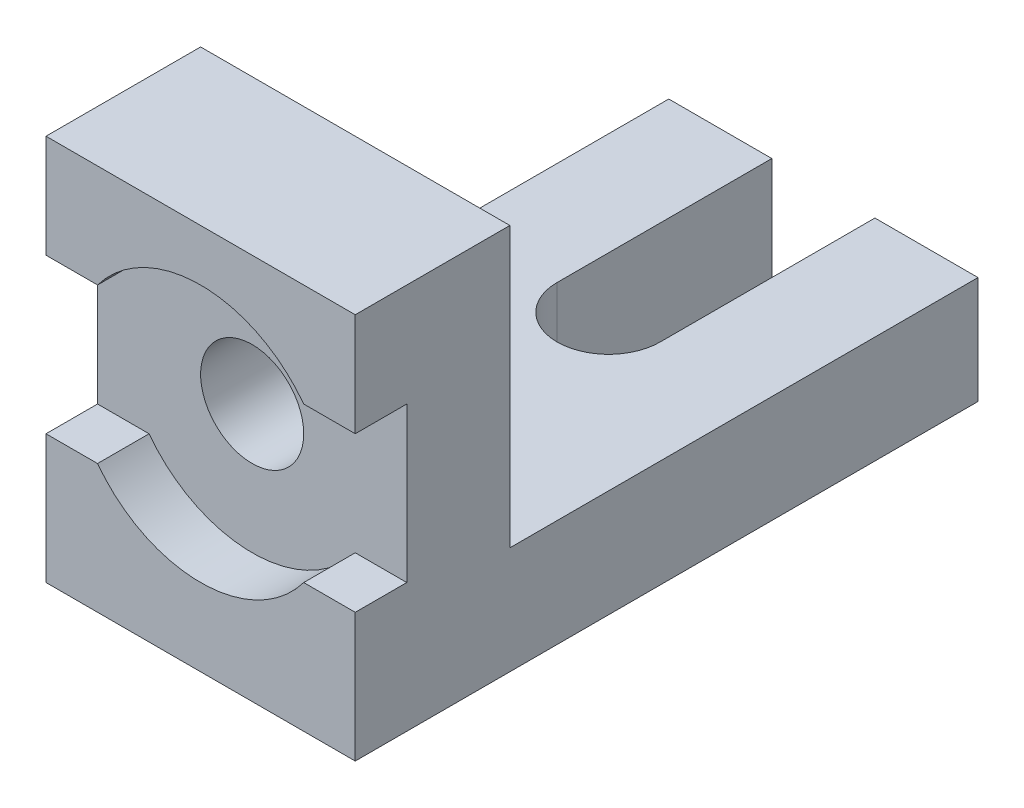
ISO-10303-21;
HEADER;
FILE_DESCRIPTION(('STEP AP214'),'2;1');
FILE_NAME('part.step','',(''),(''),'','','');
FILE_SCHEMA(('AUTOMOTIVE_DESIGN { 1 0 10303 214 1 1 1 1 }'));
ENDSEC;
DATA;
#1=APPLICATION_CONTEXT('core data for automotive mechanical design processes');
#2=APPLICATION_PROTOCOL_DEFINITION('international standard','automotive_design',2000,#1);
#3=PRODUCT_CONTEXT('',#1,'mechanical');
#4=PRODUCT('Part','Part','',(#3));
#5=PRODUCT_RELATED_PRODUCT_CATEGORY('part','',(#4));
#6=PRODUCT_DEFINITION_FORMATION('','',#4);
#7=PRODUCT_DEFINITION_CONTEXT('part definition',#1,'design');
#8=PRODUCT_DEFINITION('design','',#6,#7);
#9=PRODUCT_DEFINITION_SHAPE('','',#8);
#10=(LENGTH_UNIT() NAMED_UNIT(*) SI_UNIT(.MILLI.,.METRE.));
#11=(NAMED_UNIT(*) PLANE_ANGLE_UNIT() SI_UNIT($,.RADIAN.));
#12=(NAMED_UNIT(*) SI_UNIT($,.STERADIAN.) SOLID_ANGLE_UNIT());
#13=UNCERTAINTY_MEASURE_WITH_UNIT(LENGTH_MEASURE(1.E-05),#10,'distance_accuracy_value','');
#14=(GEOMETRIC_REPRESENTATION_CONTEXT(3) GLOBAL_UNCERTAINTY_ASSIGNED_CONTEXT((#13)) GLOBAL_UNIT_ASSIGNED_CONTEXT((#10,
#11,#12)) REPRESENTATION_CONTEXT('',''));
#15=CARTESIAN_POINT('',(0.,0.,0.));
#16=DIRECTION('',(0.,0.,1.));
#17=DIRECTION('',(1.,0.,0.));
#18=AXIS2_PLACEMENT_3D('',#15,#16,#17);
#19=CARTESIAN_POINT('',(-36.,25.,72.5));
#20=DIRECTION('',(0.,0.,-1.));
#21=DIRECTION('',(-1.,0.,0.));
#22=AXIS2_PLACEMENT_3D('',#19,#20,#21);
#23=PLANE('',#22);
#24=DIRECTION('',(0.,-1.,0.));
#25=VECTOR('',#24,1.);
#26=CARTESIAN_POINT('',(-36.,25.,72.5));
#27=LINE('',#26,#25);
#28=CARTESIAN_POINT('',(-36.,90.,72.5));
#29=VERTEX_POINT('',#28);
#30=CARTESIAN_POINT('',(-36.,66.,72.5));
#31=VERTEX_POINT('',#30);
#32=EDGE_CURVE('E288',#29,#31,#27,.T.);
#33=ORIENTED_EDGE('',*,*,#32,.T.);
#34=DIRECTION('',(-1.,0.,0.));
#35=VECTOR('',#34,1.);
#36=CARTESIAN_POINT('',(0.,66.,72.5));
#37=LINE('',#36,#35);
#38=CARTESIAN_POINT('',(-24.,66.,72.5));
#39=VERTEX_POINT('',#38);
#40=EDGE_CURVE('E183',#39,#31,#37,.T.);
#41=ORIENTED_EDGE('',*,*,#40,.F.);
#42=CARTESIAN_POINT('',(0.,48.,72.5));
#43=DIRECTION('',(0.,0.,1.));
#44=DIRECTION('',(1.,0.,0.));
#45=AXIS2_PLACEMENT_3D('',#42,#43,#44);
#46=CIRCLE('',#45,30.);
#47=CARTESIAN_POINT('',(24.,66.,72.5));
#48=VERTEX_POINT('',#47);
#49=EDGE_CURVE('E190',#48,#39,#46,.T.);
#50=ORIENTED_EDGE('',*,*,#49,.F.);
#51=DIRECTION('',(-1.,0.,0.));
#52=VECTOR('',#51,1.);
#53=CARTESIAN_POINT('',(0.,66.,72.5));
#54=LINE('',#53,#52);
#55=CARTESIAN_POINT('',(36.,66.,72.5));
#56=VERTEX_POINT('',#55);
#57=EDGE_CURVE('E211',#56,#48,#54,.T.);
#58=ORIENTED_EDGE('',*,*,#57,.F.);
#59=DIRECTION('',(0.,-1.,0.));
#60=VECTOR('',#59,1.);
#61=CARTESIAN_POINT('',(36.,25.,72.5));
#62=LINE('',#61,#60);
#63=CARTESIAN_POINT('',(36.,90.,72.5));
#64=VERTEX_POINT('',#63);
#65=EDGE_CURVE('E287',#64,#56,#62,.T.);
#66=ORIENTED_EDGE('',*,*,#65,.F.);
#67=DIRECTION('',(1.,0.,0.));
#68=VECTOR('',#67,1.);
#69=CARTESIAN_POINT('',(-36.,90.,72.5));
#70=LINE('',#69,#68);
#71=EDGE_CURVE('E232',#29,#64,#70,.T.);
#72=ORIENTED_EDGE('',*,*,#71,.F.);
#73=EDGE_LOOP('',(#33,#41,#50,#58,#66,#72));
#74=FACE_BOUND('',#73,.T.);
#75=ADVANCED_FACE('F39',(#74),#23,.F.);
#76=CARTESIAN_POINT('',(36.,25.,-72.5));
#77=DIRECTION('',(0.,0.,1.));
#78=DIRECTION('',(1.,0.,0.));
#79=AXIS2_PLACEMENT_3D('',#76,#77,#78);
#80=PLANE('',#79);
#81=DIRECTION('',(-1.,0.,0.));
#82=VECTOR('',#81,1.);
#83=CARTESIAN_POINT('',(36.,25.,-72.5));
#84=LINE('',#83,#82);
#85=CARTESIAN_POINT('',(-12.,25.,-72.5));
#86=VERTEX_POINT('',#85);
#87=CARTESIAN_POINT('',(-36.,25.,-72.5));
#88=VERTEX_POINT('',#87);
#89=EDGE_CURVE('E268',#86,#88,#84,.T.);
#90=ORIENTED_EDGE('',*,*,#89,.F.);
#91=DIRECTION('',(0.,1.,0.));
#92=VECTOR('',#91,1.);
#93=CARTESIAN_POINT('',(-12.,-25.,-72.5));
#94=LINE('',#93,#92);
#95=CARTESIAN_POINT('',(-12.,0.,-72.5));
#96=VERTEX_POINT('',#95);
#97=EDGE_CURVE('E257',#96,#86,#94,.T.);
#98=ORIENTED_EDGE('',*,*,#97,.F.);
#99=DIRECTION('',(-1.,0.,0.));
#100=VECTOR('',#99,1.);
#101=CARTESIAN_POINT('',(36.,0.,-72.5));
#102=LINE('',#101,#100);
#103=CARTESIAN_POINT('',(-36.,0.,-72.5));
#104=VERTEX_POINT('',#103);
#105=EDGE_CURVE('E280',#96,#104,#102,.T.);
#106=ORIENTED_EDGE('',*,*,#105,.T.);
#107=DIRECTION('',(0.,-1.,0.));
#108=VECTOR('',#107,1.);
#109=CARTESIAN_POINT('',(-36.,25.,-72.5));
#110=LINE('',#109,#108);
#111=EDGE_CURVE('E291',#88,#104,#110,.T.);
#112=ORIENTED_EDGE('',*,*,#111,.F.);
#113=EDGE_LOOP('',(#90,#98,#106,#112));
#114=FACE_BOUND('',#113,.T.);
#115=ADVANCED_FACE('F338',(#114),#80,.F.);
#116=CARTESIAN_POINT('',(36.,25.,0.));
#117=DIRECTION('',(-1.,0.,0.));
#118=DIRECTION('',(0.,0.,1.));
#119=AXIS2_PLACEMENT_3D('',#116,#117,#118);
#120=PLANE('',#119);
#121=ORIENTED_EDGE('',*,*,#65,.T.);
#122=DIRECTION('',(0.,0.,1.));
#123=VECTOR('',#122,1.);
#124=CARTESIAN_POINT('',(36.,66.,60.5));
#125=LINE('',#124,#123);
#126=CARTESIAN_POINT('',(36.,66.,60.5));
#127=VERTEX_POINT('',#126);
#128=EDGE_CURVE('E223',#127,#56,#125,.T.);
#129=ORIENTED_EDGE('',*,*,#128,.F.);
#130=DIRECTION('',(0.,1.,0.));
#131=VECTOR('',#130,1.);
#132=CARTESIAN_POINT('',(36.,0.,60.5));
#133=LINE('',#132,#131);
#134=CARTESIAN_POINT('',(36.,30.,60.5));
#135=VERTEX_POINT('',#134);
#136=EDGE_CURVE('E191',#135,#127,#133,.T.);
#137=ORIENTED_EDGE('',*,*,#136,.F.);
#138=DIRECTION('',(0.,0.,1.));
#139=VECTOR('',#138,1.);
#140=CARTESIAN_POINT('',(36.,30.,60.5));
#141=LINE('',#140,#139);
#142=CARTESIAN_POINT('',(36.,30.,72.5));
#143=VERTEX_POINT('',#142);
#144=EDGE_CURVE('E230',#135,#143,#141,.T.);
#145=ORIENTED_EDGE('',*,*,#144,.T.);
#146=CARTESIAN_POINT('',(36.,0.,72.5));
#147=VERTEX_POINT('',#146);
#148=EDGE_CURVE('E274',#143,#147,#62,.T.);
#149=ORIENTED_EDGE('',*,*,#148,.T.);
#150=DIRECTION('',(0.,0.,-1.));
#151=VECTOR('',#150,1.);
#152=CARTESIAN_POINT('',(36.,0.,0.));
#153=LINE('',#152,#151);
#154=CARTESIAN_POINT('',(36.,0.,-72.5));
#155=VERTEX_POINT('',#154);
#156=EDGE_CURVE('E259',#147,#155,#153,.T.);
#157=ORIENTED_EDGE('',*,*,#156,.T.);
#158=DIRECTION('',(0.,-1.,0.));
#159=VECTOR('',#158,1.);
#160=CARTESIAN_POINT('',(36.,25.,-72.5));
#161=LINE('',#160,#159);
#162=CARTESIAN_POINT('',(36.,25.,-72.5));
#163=VERTEX_POINT('',#162);
#164=EDGE_CURVE('E297',#163,#155,#161,.T.);
#165=ORIENTED_EDGE('',*,*,#164,.F.);
#166=DIRECTION('',(0.,0.,-1.));
#167=VECTOR('',#166,1.);
#168=CARTESIAN_POINT('',(36.,25.,72.5));
#169=LINE('',#168,#167);
#170=CARTESIAN_POINT('',(36.,25.,36.5));
#171=VERTEX_POINT('',#170);
#172=EDGE_CURVE('E266',#171,#163,#169,.T.);
#173=ORIENTED_EDGE('',*,*,#172,.F.);
#174=DIRECTION('',(0.,-1.,0.));
#175=VECTOR('',#174,1.);
#176=CARTESIAN_POINT('',(36.,90.,36.5));
#177=LINE('',#176,#175);
#178=CARTESIAN_POINT('',(36.,90.,36.5));
#179=VERTEX_POINT('',#178);
#180=EDGE_CURVE('E241',#179,#171,#177,.T.);
#181=ORIENTED_EDGE('',*,*,#180,.F.);
#182=DIRECTION('',(0.,0.,-1.));
#183=VECTOR('',#182,1.);
#184=CARTESIAN_POINT('',(36.,90.,72.5));
#185=LINE('',#184,#183);
#186=EDGE_CURVE('E231',#64,#179,#185,.T.);
#187=ORIENTED_EDGE('',*,*,#186,.F.);
#188=EDGE_LOOP('',(#121,#129,#137,#145,#149,#157,#165,#173,#181,#187));
#189=FACE_BOUND('',#188,.T.);
#190=ADVANCED_FACE('F41',(#189),#120,.F.);
#191=CARTESIAN_POINT('',(12.,0.,-72.5));
#192=VERTEX_POINT('',#191);
#193=EDGE_CURVE('E279',#155,#192,#102,.T.);
#194=ORIENTED_EDGE('',*,*,#193,.T.);
#195=DIRECTION('',(0.,1.,0.));
#196=VECTOR('',#195,1.);
#197=CARTESIAN_POINT('',(12.,-25.,-72.5));
#198=LINE('',#197,#196);
#199=CARTESIAN_POINT('',(12.,25.,-72.5));
#200=VERTEX_POINT('',#199);
#201=EDGE_CURVE('E265',#192,#200,#198,.T.);
#202=ORIENTED_EDGE('',*,*,#201,.T.);
#203=EDGE_CURVE('E269',#163,#200,#84,.T.);
#204=ORIENTED_EDGE('',*,*,#203,.F.);
#205=ORIENTED_EDGE('',*,*,#164,.T.);
#206=EDGE_LOOP('',(#194,#202,#204,#205));
#207=FACE_BOUND('',#206,.T.);
#208=ADVANCED_FACE('F325',(#207),#80,.F.);
#209=CARTESIAN_POINT('',(-36.,25.,-72.5));
#210=DIRECTION('',(1.,0.,0.));
#211=DIRECTION('',(0.,0.,-1.));
#212=AXIS2_PLACEMENT_3D('',#209,#210,#211);
#213=PLANE('',#212);
#214=CARTESIAN_POINT('',(-36.,30.,72.5));
#215=VERTEX_POINT('',#214);
#216=CARTESIAN_POINT('',(-36.,0.,72.5));
#217=VERTEX_POINT('',#216);
#218=EDGE_CURVE('E286',#215,#217,#27,.T.);
#219=ORIENTED_EDGE('',*,*,#218,.F.);
#220=DIRECTION('',(0.,0.,1.));
#221=VECTOR('',#220,1.);
#222=CARTESIAN_POINT('',(-36.,30.,60.5));
#223=LINE('',#222,#221);
#224=CARTESIAN_POINT('',(-36.,30.,60.5));
#225=VERTEX_POINT('',#224);
#226=EDGE_CURVE('E216',#225,#215,#223,.T.);
#227=ORIENTED_EDGE('',*,*,#226,.F.);
#228=DIRECTION('',(0.,-1.,0.));
#229=VECTOR('',#228,1.);
#230=CARTESIAN_POINT('',(-36.,0.,60.5));
#231=LINE('',#230,#229);
#232=CARTESIAN_POINT('',(-36.,66.,60.5));
#233=VERTEX_POINT('',#232);
#234=EDGE_CURVE('E172',#233,#225,#231,.T.);
#235=ORIENTED_EDGE('',*,*,#234,.F.);
#236=DIRECTION('',(0.,0.,1.));
#237=VECTOR('',#236,1.);
#238=CARTESIAN_POINT('',(-36.,66.,60.5));
#239=LINE('',#238,#237);
#240=EDGE_CURVE('E217',#233,#31,#239,.T.);
#241=ORIENTED_EDGE('',*,*,#240,.T.);
#242=ORIENTED_EDGE('',*,*,#32,.F.);
#243=DIRECTION('',(0.,0.,1.));
#244=VECTOR('',#243,1.);
#245=CARTESIAN_POINT('',(-36.,90.,36.5));
#246=LINE('',#245,#244);
#247=CARTESIAN_POINT('',(-36.,90.,36.5));
#248=VERTEX_POINT('',#247);
#249=EDGE_CURVE('E236',#248,#29,#246,.T.);
#250=ORIENTED_EDGE('',*,*,#249,.F.);
#251=DIRECTION('',(0.,-1.,0.));
#252=VECTOR('',#251,1.);
#253=CARTESIAN_POINT('',(-36.,90.,36.5));
#254=LINE('',#253,#252);
#255=CARTESIAN_POINT('',(-36.,25.,36.5));
#256=VERTEX_POINT('',#255);
#257=EDGE_CURVE('E242',#248,#256,#254,.T.);
#258=ORIENTED_EDGE('',*,*,#257,.T.);
#259=DIRECTION('',(0.,0.,1.));
#260=VECTOR('',#259,1.);
#261=CARTESIAN_POINT('',(-36.,25.,-72.5));
#262=LINE('',#261,#260);
#263=EDGE_CURVE('E272',#88,#256,#262,.T.);
#264=ORIENTED_EDGE('',*,*,#263,.F.);
#265=ORIENTED_EDGE('',*,*,#111,.T.);
#266=DIRECTION('',(0.,0.,1.));
#267=VECTOR('',#266,1.);
#268=CARTESIAN_POINT('',(-36.,0.,-72.5));
#269=LINE('',#268,#267);
#270=EDGE_CURVE('E282',#104,#217,#269,.T.);
#271=ORIENTED_EDGE('',*,*,#270,.T.);
#272=EDGE_LOOP('',(#219,#227,#235,#241,#242,#250,#258,#264,#265,#271));
#273=FACE_BOUND('',#272,.T.);
#274=ADVANCED_FACE('F331',(#273),#213,.F.);
#275=CARTESIAN_POINT('',(0.,48.,72.5));
#276=DIRECTION('',(0.,0.,1.));
#277=DIRECTION('',(1.,0.,0.));
#278=AXIS2_PLACEMENT_3D('',#275,#276,#277);
#279=CIRCLE('',#278,30.);
#280=CARTESIAN_POINT('',(-24.,30.,72.5));
#281=VERTEX_POINT('',#280);
#282=CARTESIAN_POINT('',(24.,30.,72.5));
#283=VERTEX_POINT('',#282);
#284=EDGE_CURVE('E210',#281,#283,#279,.T.);
#285=ORIENTED_EDGE('',*,*,#284,.F.);
#286=DIRECTION('',(1.,0.,0.));
#287=VECTOR('',#286,1.);
#288=CARTESIAN_POINT('',(0.,30.,72.5));
#289=LINE('',#288,#287);
#290=EDGE_CURVE('E53',#215,#281,#289,.T.);
#291=ORIENTED_EDGE('',*,*,#290,.F.);
#292=ORIENTED_EDGE('',*,*,#218,.T.);
#293=DIRECTION('',(1.,0.,0.));
#294=VECTOR('',#293,1.);
#295=CARTESIAN_POINT('',(-36.,0.,72.5));
#296=LINE('',#295,#294);
#297=EDGE_CURVE('E267',#217,#147,#296,.T.);
#298=ORIENTED_EDGE('',*,*,#297,.T.);
#299=ORIENTED_EDGE('',*,*,#148,.F.);
#300=DIRECTION('',(1.,0.,0.));
#301=VECTOR('',#300,1.);
#302=CARTESIAN_POINT('',(0.,30.,72.5));
#303=LINE('',#302,#301);
#304=EDGE_CURVE('E207',#283,#143,#303,.T.);
#305=ORIENTED_EDGE('',*,*,#304,.F.);
#306=EDGE_LOOP('',(#285,#291,#292,#298,#299,#305));
#307=FACE_BOUND('',#306,.T.);
#308=ADVANCED_FACE('F329',(#307),#23,.F.);
#309=CARTESIAN_POINT('',(0.,25.,0.));
#310=DIRECTION('',(0.,1.,0.));
#311=DIRECTION('',(0.,0.,1.));
#312=AXIS2_PLACEMENT_3D('',#309,#310,#311);
#313=PLANE('',#312);
#314=DIRECTION('',(-1.,0.,0.));
#315=VECTOR('',#314,1.);
#316=CARTESIAN_POINT('',(36.,25.,36.5));
#317=LINE('',#316,#315);
#318=EDGE_CURVE('E65',#171,#256,#317,.T.);
#319=ORIENTED_EDGE('',*,*,#318,.F.);
#320=ORIENTED_EDGE('',*,*,#172,.T.);
#321=ORIENTED_EDGE('',*,*,#203,.T.);
#322=DIRECTION('',(0.,0.,-1.));
#323=VECTOR('',#322,1.);
#324=CARTESIAN_POINT('',(12.,25.,-22.5));
#325=LINE('',#324,#323);
#326=CARTESIAN_POINT('',(12.,25.,-22.5));
#327=VERTEX_POINT('',#326);
#328=EDGE_CURVE('E253',#327,#200,#325,.T.);
#329=ORIENTED_EDGE('',*,*,#328,.F.);
#330=CARTESIAN_POINT('',(0.,25.,-22.5));
#331=DIRECTION('',(0.,1.,0.));
#332=DIRECTION('',(0.,0.,1.));
#333=AXIS2_PLACEMENT_3D('',#330,#331,#332);
#334=CIRCLE('',#333,12.);
#335=CARTESIAN_POINT('',(-12.,25.,-22.5));
#336=VERTEX_POINT('',#335);
#337=EDGE_CURVE('E249',#336,#327,#334,.T.);
#338=ORIENTED_EDGE('',*,*,#337,.F.);
#339=DIRECTION('',(0.,0.,1.));
#340=VECTOR('',#339,1.);
#341=CARTESIAN_POINT('',(-12.,25.,-22.5));
#342=LINE('',#341,#340);
#343=EDGE_CURVE('E251',#86,#336,#342,.T.);
#344=ORIENTED_EDGE('',*,*,#343,.F.);
#345=ORIENTED_EDGE('',*,*,#89,.T.);
#346=ORIENTED_EDGE('',*,*,#263,.T.);
#347=EDGE_LOOP('',(#319,#320,#321,#329,#338,#344,#345,#346));
#348=FACE_BOUND('',#347,.T.);
#349=ADVANCED_FACE('F320',(#348),#313,.T.);
#350=CARTESIAN_POINT('',(0.,0.,0.));
#351=DIRECTION('',(0.,1.,0.));
#352=DIRECTION('',(0.,0.,1.));
#353=AXIS2_PLACEMENT_3D('',#350,#351,#352);
#354=PLANE('',#353);
#355=ORIENTED_EDGE('',*,*,#105,.F.);
#356=DIRECTION('',(0.,0.,1.));
#357=VECTOR('',#356,1.);
#358=CARTESIAN_POINT('',(-12.,0.,0.));
#359=LINE('',#358,#357);
#360=CARTESIAN_POINT('',(-12.,0.,-22.5));
#361=VERTEX_POINT('',#360);
#362=EDGE_CURVE('E11',#96,#361,#359,.T.);
#363=ORIENTED_EDGE('',*,*,#362,.T.);
#364=CARTESIAN_POINT('',(0.,0.,-22.5));
#365=DIRECTION('',(0.,1.,0.));
#366=DIRECTION('',(0.,0.,1.));
#367=AXIS2_PLACEMENT_3D('',#364,#365,#366);
#368=CIRCLE('',#367,12.);
#369=CARTESIAN_POINT('',(12.,0.,-22.5));
#370=VERTEX_POINT('',#369);
#371=EDGE_CURVE('E50',#361,#370,#368,.T.);
#372=ORIENTED_EDGE('',*,*,#371,.T.);
#373=DIRECTION('',(0.,0.,-1.));
#374=VECTOR('',#373,1.);
#375=CARTESIAN_POINT('',(12.,0.,0.));
#376=LINE('',#375,#374);
#377=EDGE_CURVE('E299',#370,#192,#376,.T.);
#378=ORIENTED_EDGE('',*,*,#377,.T.);
#379=ORIENTED_EDGE('',*,*,#193,.F.);
#380=ORIENTED_EDGE('',*,*,#156,.F.);
#381=ORIENTED_EDGE('',*,*,#297,.F.);
#382=ORIENTED_EDGE('',*,*,#270,.F.);
#383=EDGE_LOOP('',(#355,#363,#372,#378,#379,#380,#381,#382));
#384=FACE_BOUND('',#383,.T.);
#385=ADVANCED_FACE('F301',(#384),#354,.F.);
#386=CARTESIAN_POINT('',(0.,-25.,-22.5));
#387=DIRECTION('',(0.,1.,0.));
#388=DIRECTION('',(0.,0.,1.));
#389=AXIS2_PLACEMENT_3D('',#386,#387,#388);
#390=CYLINDRICAL_SURFACE('',#389,12.);
#391=DIRECTION('',(0.,1.,0.));
#392=VECTOR('',#391,1.);
#393=CARTESIAN_POINT('',(-12.,-25.,-22.5));
#394=LINE('',#393,#392);
#395=EDGE_CURVE('E260',#361,#336,#394,.T.);
#396=ORIENTED_EDGE('',*,*,#395,.T.);
#397=ORIENTED_EDGE('',*,*,#337,.T.);
#398=DIRECTION('',(0.,1.,0.));
#399=VECTOR('',#398,1.);
#400=CARTESIAN_POINT('',(12.,-25.,-22.5));
#401=LINE('',#400,#399);
#402=EDGE_CURVE('E258',#370,#327,#401,.T.);
#403=ORIENTED_EDGE('',*,*,#402,.F.);
#404=ORIENTED_EDGE('',*,*,#371,.F.);
#405=EDGE_LOOP('',(#396,#397,#403,#404));
#406=FACE_BOUND('',#405,.T.);
#407=ADVANCED_FACE('F310',(#406),#390,.F.);
#408=CARTESIAN_POINT('',(-12.,-25.,-22.5));
#409=DIRECTION('',(-1.,0.,0.));
#410=DIRECTION('',(0.,0.,1.));
#411=AXIS2_PLACEMENT_3D('',#408,#409,#410);
#412=PLANE('',#411);
#413=ORIENTED_EDGE('',*,*,#97,.T.);
#414=ORIENTED_EDGE('',*,*,#343,.T.);
#415=ORIENTED_EDGE('',*,*,#395,.F.);
#416=ORIENTED_EDGE('',*,*,#362,.F.);
#417=EDGE_LOOP('',(#413,#414,#415,#416));
#418=FACE_BOUND('',#417,.T.);
#419=ADVANCED_FACE('F313',(#418),#412,.F.);
#420=CARTESIAN_POINT('',(12.,-25.,-22.5));
#421=DIRECTION('',(1.,0.,0.));
#422=DIRECTION('',(0.,0.,-1.));
#423=AXIS2_PLACEMENT_3D('',#420,#421,#422);
#424=PLANE('',#423);
#425=ORIENTED_EDGE('',*,*,#402,.T.);
#426=ORIENTED_EDGE('',*,*,#328,.T.);
#427=ORIENTED_EDGE('',*,*,#201,.F.);
#428=ORIENTED_EDGE('',*,*,#377,.F.);
#429=EDGE_LOOP('',(#425,#426,#427,#428));
#430=FACE_BOUND('',#429,.T.);
#431=ADVANCED_FACE('F319',(#430),#424,.F.);
#432=CARTESIAN_POINT('',(36.,90.,36.5));
#433=DIRECTION('',(0.,0.,1.));
#434=DIRECTION('',(1.,0.,0.));
#435=AXIS2_PLACEMENT_3D('',#432,#433,#434);
#436=PLANE('',#435);
#437=CARTESIAN_POINT('',(0.,48.,36.5));
#438=DIRECTION('',(0.,0.,1.));
#439=DIRECTION('',(1.,0.,0.));
#440=AXIS2_PLACEMENT_3D('',#437,#438,#439);
#441=CIRCLE('',#440,12.);
#442=CARTESIAN_POINT('',(12.,48.,36.5));
#443=VERTEX_POINT('',#442);
#444=EDGE_CURVE('E186',#443,#443,#441,.T.);
#445=ORIENTED_EDGE('',*,*,#444,.T.);
#446=EDGE_LOOP('',(#445));
#447=FACE_BOUND('',#446,.T.);
#448=ORIENTED_EDGE('',*,*,#318,.T.);
#449=ORIENTED_EDGE('',*,*,#257,.F.);
#450=DIRECTION('',(-1.,0.,0.));
#451=VECTOR('',#450,1.);
#452=CARTESIAN_POINT('',(36.,90.,36.5));
#453=LINE('',#452,#451);
#454=EDGE_CURVE('E237',#179,#248,#453,.T.);
#455=ORIENTED_EDGE('',*,*,#454,.F.);
#456=ORIENTED_EDGE('',*,*,#180,.T.);
#457=EDGE_LOOP('',(#448,#449,#455,#456));
#458=FACE_BOUND('',#457,.T.);
#459=ADVANCED_FACE('F342',(#447,#458),#436,.F.);
#460=CARTESIAN_POINT('',(0.,90.,0.));
#461=DIRECTION('',(0.,1.,0.));
#462=DIRECTION('',(0.,0.,1.));
#463=AXIS2_PLACEMENT_3D('',#460,#461,#462);
#464=PLANE('',#463);
#465=ORIENTED_EDGE('',*,*,#71,.T.);
#466=ORIENTED_EDGE('',*,*,#186,.T.);
#467=ORIENTED_EDGE('',*,*,#454,.T.);
#468=ORIENTED_EDGE('',*,*,#249,.T.);
#469=EDGE_LOOP('',(#465,#466,#467,#468));
#470=FACE_BOUND('',#469,.T.);
#471=ADVANCED_FACE('F350',(#470),#464,.T.);
#472=CARTESIAN_POINT('',(0.,30.,60.5));
#473=DIRECTION('',(0.,-1.,0.));
#474=DIRECTION('',(0.,0.,-1.));
#475=AXIS2_PLACEMENT_3D('',#472,#473,#474);
#476=PLANE('',#475);
#477=ORIENTED_EDGE('',*,*,#290,.T.);
#478=DIRECTION('',(0.,0.,1.));
#479=VECTOR('',#478,1.);
#480=CARTESIAN_POINT('',(-24.,30.,60.5));
#481=LINE('',#480,#479);
#482=CARTESIAN_POINT('',(-24.,30.,60.5));
#483=VERTEX_POINT('',#482);
#484=EDGE_CURVE('E161',#483,#281,#481,.T.);
#485=ORIENTED_EDGE('',*,*,#484,.F.);
#486=DIRECTION('',(1.,0.,0.));
#487=VECTOR('',#486,1.);
#488=CARTESIAN_POINT('',(0.,30.,60.5));
#489=LINE('',#488,#487);
#490=EDGE_CURVE('E164',#225,#483,#489,.T.);
#491=ORIENTED_EDGE('',*,*,#490,.F.);
#492=ORIENTED_EDGE('',*,*,#226,.T.);
#493=EDGE_LOOP('',(#477,#485,#491,#492));
#494=FACE_BOUND('',#493,.T.);
#495=ADVANCED_FACE('F162',(#494),#476,.F.);
#496=CARTESIAN_POINT('',(0.,66.,60.5));
#497=DIRECTION('',(0.,1.,0.));
#498=DIRECTION('',(0.,0.,1.));
#499=AXIS2_PLACEMENT_3D('',#496,#497,#498);
#500=PLANE('',#499);
#501=ORIENTED_EDGE('',*,*,#40,.T.);
#502=ORIENTED_EDGE('',*,*,#240,.F.);
#503=DIRECTION('',(-1.,0.,0.));
#504=VECTOR('',#503,1.);
#505=CARTESIAN_POINT('',(0.,66.,60.5));
#506=LINE('',#505,#504);
#507=CARTESIAN_POINT('',(-24.,66.,60.5));
#508=VERTEX_POINT('',#507);
#509=EDGE_CURVE('E201',#508,#233,#506,.T.);
#510=ORIENTED_EDGE('',*,*,#509,.F.);
#511=DIRECTION('',(0.,0.,1.));
#512=VECTOR('',#511,1.);
#513=CARTESIAN_POINT('',(-24.,66.,60.5));
#514=LINE('',#513,#512);
#515=EDGE_CURVE('E222',#508,#39,#514,.T.);
#516=ORIENTED_EDGE('',*,*,#515,.T.);
#517=EDGE_LOOP('',(#501,#502,#510,#516));
#518=FACE_BOUND('',#517,.T.);
#519=ADVANCED_FACE('F424',(#518),#500,.F.);
#520=CARTESIAN_POINT('',(0.,48.,60.5));
#521=DIRECTION('',(0.,0.,1.));
#522=DIRECTION('',(1.,0.,0.));
#523=AXIS2_PLACEMENT_3D('',#520,#521,#522);
#524=CYLINDRICAL_SURFACE('',#523,30.);
#525=ORIENTED_EDGE('',*,*,#49,.T.);
#526=ORIENTED_EDGE('',*,*,#515,.F.);
#527=CARTESIAN_POINT('',(0.,48.,60.5));
#528=DIRECTION('',(0.,0.,1.));
#529=DIRECTION('',(1.,0.,0.));
#530=AXIS2_PLACEMENT_3D('',#527,#528,#529);
#531=CIRCLE('',#530,30.);
#532=CARTESIAN_POINT('',(24.,66.,60.5));
#533=VERTEX_POINT('',#532);
#534=EDGE_CURVE('E199',#533,#508,#531,.T.);
#535=ORIENTED_EDGE('',*,*,#534,.F.);
#536=DIRECTION('',(0.,0.,1.));
#537=VECTOR('',#536,1.);
#538=CARTESIAN_POINT('',(24.,66.,60.5));
#539=LINE('',#538,#537);
#540=EDGE_CURVE('E224',#533,#48,#539,.T.);
#541=ORIENTED_EDGE('',*,*,#540,.T.);
#542=EDGE_LOOP('',(#525,#526,#535,#541));
#543=FACE_BOUND('',#542,.T.);
#544=ADVANCED_FACE('F433',(#543),#524,.F.);
#545=CARTESIAN_POINT('',(0.,66.,60.5));
#546=DIRECTION('',(0.,1.,0.));
#547=DIRECTION('',(0.,0.,1.));
#548=AXIS2_PLACEMENT_3D('',#545,#546,#547);
#549=PLANE('',#548);
#550=ORIENTED_EDGE('',*,*,#57,.T.);
#551=ORIENTED_EDGE('',*,*,#540,.F.);
#552=DIRECTION('',(-1.,0.,0.));
#553=VECTOR('',#552,1.);
#554=CARTESIAN_POINT('',(0.,66.,60.5));
#555=LINE('',#554,#553);
#556=EDGE_CURVE('E197',#127,#533,#555,.T.);
#557=ORIENTED_EDGE('',*,*,#556,.F.);
#558=ORIENTED_EDGE('',*,*,#128,.T.);
#559=EDGE_LOOP('',(#550,#551,#557,#558));
#560=FACE_BOUND('',#559,.T.);
#561=ADVANCED_FACE('F444',(#560),#549,.F.);
#562=CARTESIAN_POINT('',(0.,30.,60.5));
#563=DIRECTION('',(0.,-1.,0.));
#564=DIRECTION('',(0.,0.,-1.));
#565=AXIS2_PLACEMENT_3D('',#562,#563,#564);
#566=PLANE('',#565);
#567=ORIENTED_EDGE('',*,*,#304,.T.);
#568=ORIENTED_EDGE('',*,*,#144,.F.);
#569=DIRECTION('',(1.,0.,0.));
#570=VECTOR('',#569,1.);
#571=CARTESIAN_POINT('',(0.,30.,60.5));
#572=LINE('',#571,#570);
#573=CARTESIAN_POINT('',(24.,30.,60.5));
#574=VERTEX_POINT('',#573);
#575=EDGE_CURVE('E176',#574,#135,#572,.T.);
#576=ORIENTED_EDGE('',*,*,#575,.F.);
#577=DIRECTION('',(0.,0.,1.));
#578=VECTOR('',#577,1.);
#579=CARTESIAN_POINT('',(24.,30.,60.5));
#580=LINE('',#579,#578);
#581=EDGE_CURVE('E168',#574,#283,#580,.T.);
#582=ORIENTED_EDGE('',*,*,#581,.T.);
#583=EDGE_LOOP('',(#567,#568,#576,#582));
#584=FACE_BOUND('',#583,.T.);
#585=ADVANCED_FACE('F454',(#584),#566,.F.);
#586=CARTESIAN_POINT('',(0.,48.,60.5));
#587=DIRECTION('',(0.,0.,1.));
#588=DIRECTION('',(1.,0.,0.));
#589=AXIS2_PLACEMENT_3D('',#586,#587,#588);
#590=CYLINDRICAL_SURFACE('',#589,30.);
#591=ORIENTED_EDGE('',*,*,#284,.T.);
#592=ORIENTED_EDGE('',*,*,#581,.F.);
#593=CARTESIAN_POINT('',(0.,48.,60.5));
#594=DIRECTION('',(0.,0.,1.));
#595=DIRECTION('',(1.,0.,0.));
#596=AXIS2_PLACEMENT_3D('',#593,#594,#595);
#597=CIRCLE('',#596,30.);
#598=EDGE_CURVE('E174',#483,#574,#597,.T.);
#599=ORIENTED_EDGE('',*,*,#598,.F.);
#600=ORIENTED_EDGE('',*,*,#484,.T.);
#601=EDGE_LOOP('',(#591,#592,#599,#600));
#602=FACE_BOUND('',#601,.T.);
#603=ADVANCED_FACE('F171',(#602),#590,.F.);
#604=CARTESIAN_POINT('',(0.,0.,60.5));
#605=DIRECTION('',(0.,0.,1.));
#606=DIRECTION('',(1.,0.,0.));
#607=AXIS2_PLACEMENT_3D('',#604,#605,#606);
#608=PLANE('',#607);
#609=CARTESIAN_POINT('',(0.,48.,60.5));
#610=DIRECTION('',(0.,0.,1.));
#611=DIRECTION('',(1.,0.,0.));
#612=AXIS2_PLACEMENT_3D('',#609,#610,#611);
#613=CIRCLE('',#612,12.);
#614=CARTESIAN_POINT('',(12.,48.,60.5));
#615=VERTEX_POINT('',#614);
#616=EDGE_CURVE('E547',#615,#615,#613,.T.);
#617=ORIENTED_EDGE('',*,*,#616,.F.);
#618=EDGE_LOOP('',(#617));
#619=FACE_BOUND('',#618,.T.);
#620=ORIENTED_EDGE('',*,*,#490,.T.);
#621=ORIENTED_EDGE('',*,*,#598,.T.);
#622=ORIENTED_EDGE('',*,*,#575,.T.);
#623=ORIENTED_EDGE('',*,*,#136,.T.);
#624=ORIENTED_EDGE('',*,*,#556,.T.);
#625=ORIENTED_EDGE('',*,*,#534,.T.);
#626=ORIENTED_EDGE('',*,*,#509,.T.);
#627=ORIENTED_EDGE('',*,*,#234,.T.);
#628=EDGE_LOOP('',(#620,#621,#622,#623,#624,#625,#626,#627));
#629=FACE_BOUND('',#628,.T.);
#630=ADVANCED_FACE('F182',(#619,#629),#608,.T.);
#631=CARTESIAN_POINT('',(0.,48.,-45.5));
#632=DIRECTION('',(0.,0.,1.));
#633=DIRECTION('',(1.,0.,0.));
#634=AXIS2_PLACEMENT_3D('',#631,#632,#633);
#635=CYLINDRICAL_SURFACE('',#634,12.);
#636=ORIENTED_EDGE('',*,*,#616,.T.);
#637=EDGE_LOOP('',(#636));
#638=FACE_BOUND('',#637,.T.);
#639=ORIENTED_EDGE('',*,*,#444,.F.);
#640=EDGE_LOOP('',(#639));
#641=FACE_BOUND('',#640,.T.);
#642=ADVANCED_FACE('F476',(#638,#641),#635,.F.);
#643=CLOSED_SHELL('',(#75,#115,#190,#208,#274,#308,#349,#385,#407,#419,#431,#459,#471,#495,#519,
#544,#561,#585,#603,#630,#642));
#644=MANIFOLD_SOLID_BREP('B2',#643);
#645=ADVANCED_BREP_SHAPE_REPRESENTATION('',(#18,#644),#14);
#646=SHAPE_DEFINITION_REPRESENTATION(#9,#645);
ENDSEC;
END-ISO-10303-21;
